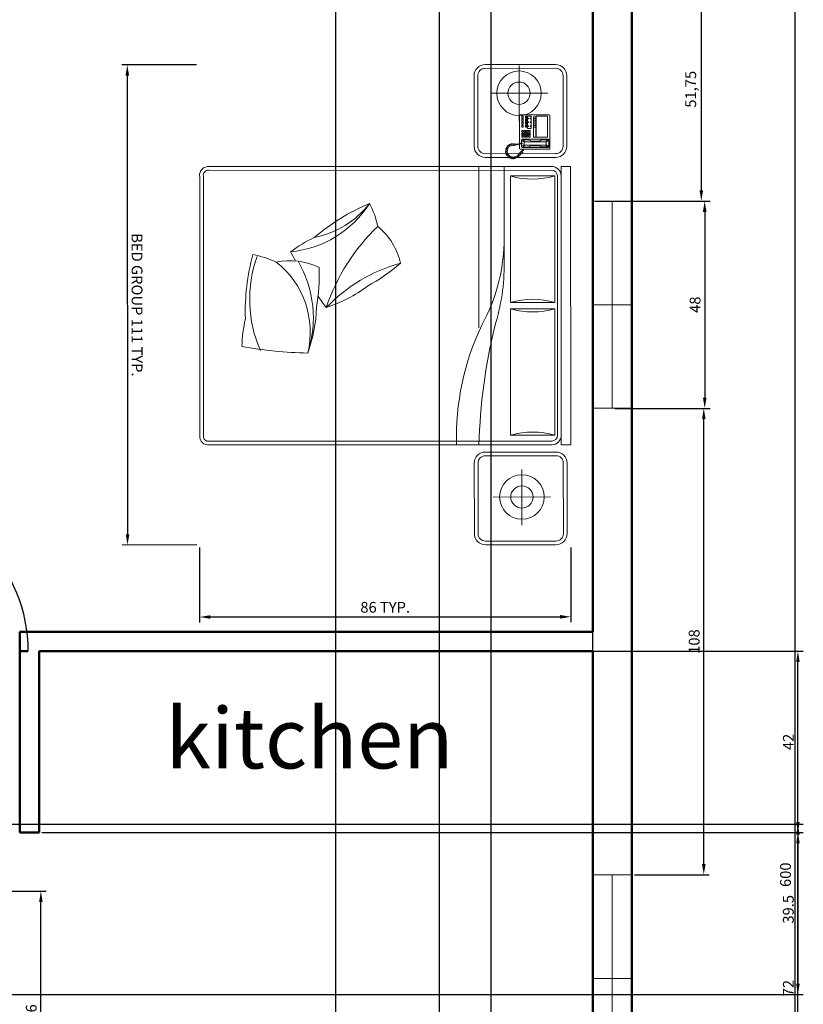
# Model space of a CAD drawing. Units: inches. Extents: x 907 to 2409, y 377 to 1163.
# Tile 7 of 9: x 1197 to 1378, y 687 to 915. Entities that reach past the tile are written whole.
import ezdxf

# ---------------------------------------------------------------- set-up
doc = ezdxf.new("R2010")
doc.units = ezdxf.units.IN
for name, color, linetype, lineweight in [('A-ANNO-DIMS', 2, 'Continuous', 18), ('A-AREA-IDEN', 7, 'Continuous', 18), ('A-DOOR', 3, 'Continuous', 25), ('A-FURN', 8, 'Continuous', 18), ('A-GLAZ', 4, 'Continuous', 18), ('A-WALL', 7, 'Continuous', 50)]:
    doc.layers.add(name, color=color, linetype=linetype, lineweight=lineweight)
doc.styles.get("Standard").update_dxf_attribs({"font": 'arial.ttf'})
doc.dimstyles.new('ISO-25', dxfattribs={"dimtxt": 2.5, "dimasz": 2.5, "dimexe": 1.25, "dimexo": 0.625, "dimtad": 1, "dimtxsty": 'Standard', "dimcen": 2.5, "dimadec": 0, "dimazin": 0, "dimtfac": 1, "dimtmove": 0, "dimatfit": 3, "dimfxl": 1, "dimarcsym": 0})

# ---------------------------------------------------------------- blocks, each defined once
blk = doc.blocks.new('A$C356F0359')
for p, q in [((0.4398, 1.9801), (0.0598, 1.9801)), ((0.5489, 2), (2.0492, 2)), ((0.5489, 1.9489), (0.5489, 2)), ((2.0492, 1.9489), (2.0492, 2)), ((2.5283, 1.9801), (2.1483, 1.9801)), ((-0.0002, 1.9201), (-0.0002, 1.5401)), ((0.0198, 1.9201), (0.0198, 1.5401)), ((0.4398, 1.9601), (0.0598, 1.9601)), ((0.4798, 1.5401), (0.4798, 1.9201)), ((0.4998, 1.5401), (0.4998, 1.9201)), ((2.0492, 1.9489), (0.5489, 1.9489)), ((1.998, 1.9289), (0.6001, 1.9289)), ((2.0883, 1.9201), (2.0883, 1.5401)), ((2.1083, 1.9201), (2.1083, 1.5401)), ((2.5283, 1.9601), (2.1483, 1.9601)), ((2.5683, 1.5401), (2.5683, 1.9201)), ((2.5883, 1.5401), (2.5883, 1.9201)), ((0.1539, 1.5681), (0.1539, 1.8777)), ((0.2725, 1.8879), (0.2702, 1.8856)), ((0.2702, 1.8856), (0.2702, 1.7279)), ((0.2725, 1.8879), (0.4531, 1.8879)), ((0.3913, 1.8753), (0.277, 1.8753)), ((0.277, 1.8753), (0.277, 1.8147)), ((0.3913, 1.8147), (0.3913, 1.8753)), ((0.4016, 1.8787), (0.4062, 1.8845)), ((0.4016, 1.7404), (0.4016, 1.8787)), ((0.4062, 1.881), (0.405, 1.8765)), ((0.405, 1.8765), (0.4153, 1.8662)), ((0.405, 1.8765), (0.405, 1.8456)), ((0.4062, 1.8845), (0.4405, 1.8845)), ((0.4108, 1.8833), (0.4062, 1.881)), ((0.4108, 1.8833), (0.4382, 1.8833)), ((0.4165, 1.8685), (0.4108, 1.8833)), ((0.4153, 1.8662), (0.4165, 1.8685)), ((0.4153, 1.8147), (0.4153, 1.8662)), ((0.4325, 1.8685), (0.4165, 1.8685)), ((0.4325, 1.8685), (0.4382, 1.8833)), ((0.4336, 1.8662), (0.4325, 1.8685)), ((0.4439, 1.8765), (0.4336, 1.8662)), ((0.4336, 1.8147), (0.4336, 1.8662)), ((0.4382, 1.8833), (0.4428, 1.881)), ((0.4405, 1.8845), (0.4462, 1.8787)), ((0.4428, 1.881), (0.4439, 1.8765)), ((0.4439, 1.8765), (0.4439, 1.8456)), ((0.4462, 1.8787), (0.4462, 1.7416)), ((0.4531, 1.8879), (0.4553, 1.8856)), ((0.4553, 1.8856), (0.4553, 1.7279)), ((0.5489, 1.8977), (0.5489, 0.0512)), ((0.5689, 1.8977), (0.5689, 0.0512)), ((2.0292, 0.0512), (2.0292, 1.8977)), ((2.0492, 0.0512), (2.0492, 1.8977)), ((2.3306, 1.5822), (2.3306, 1.8917)), ((0.277, 1.8147), (0.3913, 1.8147)), ((0.3913, 1.8125), (0.2816, 1.8125)), ((0.2816, 1.8125), (0.2816, 1.801)), ((0.2907, 1.8125), (0.2907, 1.801)), ((0.2999, 1.8125), (0.2999, 1.801)), ((0.309, 1.8125), (0.309, 1.801)), ((0.3182, 1.8125), (0.3182, 1.801)), ((0.3273, 1.8125), (0.3273, 1.801)), ((0.3365, 1.8125), (0.3365, 1.801)), ((0.3913, 1.801), (0.3913, 1.8125)), ((0.405, 1.8456), (0.4073, 1.8399)), ((0.4073, 1.8399), (0.4108, 1.8342)), ((0.4108, 1.8342), (0.4119, 1.8262)), ((0.4119, 1.8262), (0.4119, 1.8147)), ((0.4119, 1.793), (0.4119, 1.8147)), ((0.4153, 1.8147), (0.4153, 1.753)), ((0.4336, 1.8147), (0.4336, 1.753)), ((0.4382, 1.8342), (0.4371, 1.8262)), ((0.4371, 1.8262), (0.4371, 1.8147)), ((0.4371, 1.793), (0.4371, 1.8147)), ((0.4416, 1.8399), (0.4382, 1.8342)), ((0.4439, 1.8456), (0.4416, 1.8399)), ((0.277, 1.7885), (0.277, 1.7679)), ((0.3445, 1.7885), (0.277, 1.7885)), ((0.277, 1.7679), (0.3445, 1.7679)), ((0.2782, 1.7622), (0.2782, 1.7576)), ((0.2896, 1.7622), (0.2782, 1.7622)), ((0.2782, 1.7576), (0.2896, 1.7576)), ((0.2816, 1.801), (0.3913, 1.801)), ((0.2885, 1.7862), (0.2885, 1.7827)), ((0.2919, 1.7862), (0.2885, 1.7862)), ((0.2885, 1.7827), (0.2919, 1.7827)), ((0.2919, 1.7736), (0.2885, 1.7736)), ((0.2885, 1.7736), (0.2885, 1.7702)), ((0.2885, 1.7702), (0.2919, 1.7702)), ((0.2896, 1.7576), (0.2896, 1.7622)), ((0.2919, 1.7827), (0.2919, 1.7862)), ((0.2919, 1.7702), (0.2919, 1.7736)), ((0.2942, 1.7622), (0.2942, 1.7576)), ((0.3056, 1.7622), (0.2942, 1.7622)), ((0.2942, 1.7576), (0.3056, 1.7576)), ((0.3056, 1.7576), (0.3056, 1.7622)), ((0.3125, 1.7862), (0.309, 1.7862)), ((0.309, 1.7862), (0.309, 1.7827)), ((0.309, 1.7827), (0.3125, 1.7827)), ((0.3125, 1.7736), (0.309, 1.7736)), ((0.309, 1.7736), (0.309, 1.7702)), ((0.309, 1.7702), (0.3125, 1.7702)), ((0.3102, 1.7622), (0.3102, 1.7576)), ((0.3216, 1.7622), (0.3102, 1.7622)), ((0.3102, 1.7576), (0.3216, 1.7576)), ((0.3125, 1.7827), (0.3125, 1.7862)), ((0.3125, 1.7702), (0.3125, 1.7736)), ((0.3216, 1.7576), (0.3216, 1.7622)), ((0.3376, 1.7622), (0.3262, 1.7622)), ((0.3262, 1.7622), (0.3262, 1.7576)), ((0.3262, 1.7576), (0.3376, 1.7576)), ((0.333, 1.7862), (0.3296, 1.7862)), ((0.3296, 1.7862), (0.3296, 1.7827)), ((0.3296, 1.7827), (0.333, 1.7827)), ((0.333, 1.7736), (0.3296, 1.7736)), ((0.3296, 1.7736), (0.3296, 1.7702)), ((0.3296, 1.7702), (0.333, 1.7702)), ((0.333, 1.7827), (0.333, 1.7862)), ((0.333, 1.7702), (0.333, 1.7736)), ((0.3376, 1.7576), (0.3376, 1.7622)), ((0.3445, 1.7679), (0.3445, 1.7885)), ((0.3548, 1.7759), (0.3548, 1.7827)), ((0.3548, 1.7827), (0.3639, 1.7827)), ((0.3639, 1.7759), (0.3548, 1.7759)), ((0.3548, 1.7633), (0.3548, 1.7702)), ((0.3548, 1.7702), (0.3639, 1.7702)), ((0.3639, 1.7633), (0.3548, 1.7633)), ((0.3548, 1.7564), (0.3639, 1.7564)), ((0.3548, 1.7496), (0.3548, 1.7564)), ((0.3639, 1.7827), (0.3639, 1.7759)), ((0.3639, 1.7702), (0.3639, 1.7633)), ((0.3639, 1.7564), (0.3639, 1.7496)), ((0.3685, 1.7827), (0.3776, 1.7827)), ((0.3685, 1.7759), (0.3685, 1.7827)), ((0.3776, 1.7759), (0.3685, 1.7759)), ((0.3685, 1.7633), (0.3685, 1.7702)), ((0.3685, 1.7702), (0.3776, 1.7702)), ((0.3776, 1.7633), (0.3685, 1.7633)), ((0.3685, 1.7564), (0.3776, 1.7564)), ((0.3685, 1.7496), (0.3685, 1.7564)), ((0.3776, 1.7827), (0.3776, 1.7759)), ((0.3776, 1.7702), (0.3776, 1.7633)), ((0.3776, 1.7564), (0.3776, 1.7496)), ((0.3822, 1.7759), (0.3822, 1.7827)), ((0.3822, 1.7827), (0.3913, 1.7827)), ((0.3913, 1.7759), (0.3822, 1.7759)), ((0.3822, 1.7633), (0.3822, 1.7702)), ((0.3822, 1.7702), (0.3913, 1.7702)), ((0.3913, 1.7633), (0.3822, 1.7633)), ((0.3822, 1.7576), (0.3913, 1.7576)), ((0.3822, 1.7507), (0.3822, 1.7576)), ((0.3913, 1.7827), (0.3913, 1.7759)), ((0.3913, 1.7702), (0.3913, 1.7633)), ((0.3913, 1.7576), (0.3913, 1.7507)), ((0.405, 1.7736), (0.4073, 1.7793)), ((0.405, 1.7427), (0.405, 1.7736)), ((0.405, 1.7427), (0.4153, 1.753)), ((0.4073, 1.7793), (0.4108, 1.785)), ((0.4108, 1.785), (0.4119, 1.793)), ((0.4153, 1.753), (0.4165, 1.7507)), ((0.4336, 1.753), (0.4325, 1.7507)), ((0.4439, 1.7427), (0.4336, 1.753)), ((0.4382, 1.785), (0.4371, 1.793)), ((0.4416, 1.7793), (0.4382, 1.785)), ((0.4439, 1.7736), (0.4416, 1.7793)), ((0.4439, 1.7427), (0.4439, 1.7736)), ((0.3052, 1.7226), (0.0051, 1.7226)), ((0.2702, 1.7279), (0.2725, 1.7256)), ((0.4244, 1.7256), (0.2725, 1.7256)), ((0.2782, 1.745), (0.2896, 1.745)), ((0.2782, 1.7382), (0.2782, 1.745)), ((0.2896, 1.7382), (0.2782, 1.7382)), ((0.2896, 1.745), (0.2896, 1.7382)), ((0.2942, 1.745), (0.3056, 1.745)), ((0.2942, 1.7382), (0.2942, 1.745)), ((0.3056, 1.7382), (0.2942, 1.7382)), ((0.3056, 1.745), (0.3056, 1.7382)), ((0.3102, 1.745), (0.3216, 1.745)), ((0.3102, 1.7382), (0.3102, 1.745)), ((0.3216, 1.7382), (0.3102, 1.7382)), ((0.3216, 1.745), (0.3216, 1.7382)), ((0.3262, 1.7382), (0.3262, 1.745)), ((0.3262, 1.745), (0.3376, 1.745)), ((0.3376, 1.7382), (0.3262, 1.7382)), ((0.3376, 1.745), (0.3376, 1.7382)), ((0.3639, 1.7496), (0.3548, 1.7496)), ((0.3548, 1.737), (0.3548, 1.7439)), ((0.3548, 1.7439), (0.3639, 1.7439)), ((0.3639, 1.737), (0.3548, 1.737)), ((0.3639, 1.7439), (0.3639, 1.737)), ((0.3776, 1.7496), (0.3685, 1.7496)), ((0.3685, 1.737), (0.3685, 1.7439)), ((0.3685, 1.7439), (0.3776, 1.7439)), ((0.3776, 1.737), (0.3685, 1.737)), ((0.3776, 1.7439), (0.3776, 1.737)), ((0.3913, 1.7507), (0.3822, 1.7507)), ((0.3822, 1.7439), (0.3913, 1.7439)), ((0.3822, 1.737), (0.3822, 1.7439)), ((0.3913, 1.737), (0.3822, 1.737)), ((0.3913, 1.7439), (0.3913, 1.737)), ((0.4073, 1.7347), (0.4016, 1.7404)), ((0.4062, 1.7382), (0.405, 1.7427)), ((0.4108, 1.7359), (0.4062, 1.7382)), ((0.4234, 1.7347), (0.4073, 1.7347)), ((0.4165, 1.7507), (0.4108, 1.7359)), ((0.4108, 1.7359), (0.4234, 1.7359)), ((0.4325, 1.7507), (0.4165, 1.7507)), ((0.4233, 1.7393), (0.4235, 1.7294)), ((0.4268, 1.7393), (0.4233, 1.7393)), ((0.4235, 1.7294), (0.4263, 1.7179)), ((0.4263, 1.7179), (0.429, 1.707)), ((0.4274, 1.7301), (0.4268, 1.7393)), ((0.427, 1.7359), (0.4382, 1.7359)), ((0.4295, 1.6996), (0.427, 1.697)), ((0.4405, 1.7347), (0.4271, 1.7347)), ((0.429, 1.7227), (0.4274, 1.7301)), ((0.4531, 1.7256), (0.4284, 1.7256)), ((0.429, 1.707), (0.4288, 1.701)), ((0.4288, 1.701), (0.4295, 1.6996)), ((0.4318, 1.7119), (0.429, 1.7227)), ((0.4325, 1.7063), (0.4318, 1.7119)), ((0.4323, 1.7003), (0.4325, 1.7063)), ((0.4364, 1.6973), (0.4323, 1.7003)), ((0.4325, 1.7507), (0.4382, 1.7359)), ((0.4382, 1.7359), (0.4428, 1.7382)), ((0.4462, 1.7416), (0.4405, 1.7347)), ((0.4428, 1.7382), (0.4439, 1.7427)), ((0.4553, 1.7279), (0.4531, 1.7256)), ((0.4622, 1.7459), (0.4553, 1.7484)), ((0.4553, 1.7439), (0.4604, 1.7425)), ((0.4604, 1.7425), (0.465, 1.7388)), ((0.4654, 1.7427), (0.4622, 1.7459)), ((0.465, 1.7388), (0.4662, 1.7372)), ((0.4678, 1.7405), (0.4654, 1.7427)), ((0.4662, 1.7372), (0.4686, 1.7374)), ((0.4686, 1.7374), (0.4662, 1.735)), ((0.4662, 1.735), (0.4755, 1.7268)), ((0.4721, 1.7421), (0.4678, 1.7405)), ((0.4741, 1.7401), (0.4721, 1.7421)), ((0.4725, 1.7366), (0.4741, 1.7401)), ((0.4753, 1.7388), (0.4725, 1.7366)), ((0.4783, 1.7356), (0.4753, 1.7388)), ((0.4755, 1.7268), (0.4906, 1.7139)), ((0.4759, 1.729), (0.4783, 1.7356)), ((0.4821, 1.7322), (0.4759, 1.729)), ((0.4874, 1.7272), (0.4821, 1.7322)), ((0.4862, 1.7199), (0.4874, 1.7272)), ((0.4914, 1.7231), (0.4862, 1.7199)), ((0.4908, 1.7135), (0.4984, 1.6917)), ((0.4958, 1.7185), (0.4914, 1.7231)), ((0.494, 1.7135), (0.4958, 1.7185)), ((0.501, 1.7142), (0.494, 1.7135)), ((0.4964, 1.7047), (0.5031, 1.7072)), ((0.5038, 1.7049), (0.4964, 1.7047)), ((0.5005, 1.695), (0.5054, 1.6996)), ((0.5031, 1.7072), (0.501, 1.7142)), ((0.5054, 1.6996), (0.5038, 1.7049)), ((2.4819, 1.7366), (2.1818, 1.7366)), ((0.427, 1.697), (0.4265, 1.6915)), ((0.4265, 1.6915), (0.4332, 1.6903)), ((0.4332, 1.6903), (0.4267, 1.6864)), ((0.4267, 1.6864), (0.4272, 1.6801)), ((0.4272, 1.6801), (0.4346, 1.6794)), ((0.4346, 1.6794), (0.4281, 1.6744)), ((0.4281, 1.6744), (0.4311, 1.669)), ((0.4311, 1.669), (0.4381, 1.6704)), ((0.4381, 1.6704), (0.4348, 1.6639)), ((0.4348, 1.6639), (0.4383, 1.6598)), ((0.4355, 1.6919), (0.4364, 1.6973)), ((0.4367, 1.6774), (0.4355, 1.6919)), ((0.4455, 1.6663), (0.4367, 1.6774)), ((0.4383, 1.6598), (0.4436, 1.6637)), ((0.4436, 1.6637), (0.4427, 1.6575)), ((0.4427, 1.6575), (0.4471, 1.6547)), ((0.4577, 1.6598), (0.4455, 1.6663)), ((0.4471, 1.6547), (0.4526, 1.6593)), ((0.4526, 1.6593), (0.4519, 1.6517)), ((0.4519, 1.6517), (0.4568, 1.6503)), ((0.4568, 1.6503), (0.4598, 1.6565)), ((0.4716, 1.6586), (0.4577, 1.6598)), ((0.4598, 1.6565), (0.4626, 1.6503)), ((0.4626, 1.6503), (0.4665, 1.6498)), ((0.4665, 1.6498), (0.4681, 1.6565)), ((0.4681, 1.6565), (0.4707, 1.6491)), ((0.4707, 1.6491), (0.4751, 1.6503)), ((0.485, 1.6644), (0.4716, 1.6586)), ((0.4751, 1.6503), (0.4753, 1.6565)), ((0.4753, 1.6565), (0.4806, 1.6519)), ((0.4806, 1.6519), (0.4843, 1.6538)), ((0.4843, 1.6538), (0.4836, 1.6607)), ((0.4836, 1.6607), (0.4885, 1.6547)), ((0.4952, 1.6744), (0.485, 1.6644)), ((0.4885, 1.6547), (0.4922, 1.6579)), ((0.4922, 1.6579), (0.4894, 1.6642)), ((0.4894, 1.6642), (0.4959, 1.6614)), ((0.4984, 1.6917), (0.4952, 1.6744)), ((0.4957, 1.6704), (0.5024, 1.6683)), ((0.4989, 1.6642), (0.4957, 1.6704)), ((0.4959, 1.6614), (0.4989, 1.6642)), ((0.5042, 1.673), (0.4987, 1.6792)), ((0.4987, 1.6792), (0.5058, 1.679)), ((0.5068, 1.695), (0.5005, 1.695)), ((0.5008, 1.6871), (0.5079, 1.6892)), ((0.5068, 1.6836), (0.5008, 1.6871)), ((0.5024, 1.6683), (0.5042, 1.673)), ((0.5058, 1.679), (0.5068, 1.6836)), ((0.5079, 1.6892), (0.5068, 1.695)), ((0.0598, 1.5001), (0.4398, 1.5001)), ((2.1483, 1.5001), (2.5283, 1.5001)), ((0.0598, 1.4801), (0.4398, 1.4801)), ((2.1483, 1.4801), (2.5283, 1.4801)), ((0.6001, 0.02), (1.998, 0.02)), ((0.6001, 0), (1.998, 0))]:
    blk.add_line(p, q)
at = {"linetype": 'ByBlock'}
for p, q in [((0.6001, 1.9147), (1.282, 1.9147)), ((0.6001, 1.6759), (0.6001, 1.9147)), ((1.282, 1.9147), (1.282, 1.6759)), ((1.3161, 1.9147), (1.998, 1.9147)), ((1.3161, 1.6759), (1.3161, 1.9147)), ((1.998, 1.9147), (1.998, 1.6759)), ((1.282, 1.6759), (0.6001, 1.6759)), ((1.998, 1.6759), (1.3161, 1.6759)), ((1.0687, 1.6418), (0.5489, 1.6418)), ((1.4185, 1.5053), (0.5489, 1.5053))]:
    blk.add_line(p, q, dxfattribs=at)
for centre in [(0.1539, 1.7226), (2.3306, 1.7366)]:
    blk.add_circle(centre, 0.12, dxfattribs=at)
for centre in [(0.1539, 1.7226), (2.3306, 1.7366)]:
    blk.add_circle(centre, 0.06)
for centre, radius, start, end in [((0.0598, 1.9201), 0.06, 90, 180), ((0.4398, 1.9201), 0.06, 0, 90), ((2.1483, 1.9201), 0.06, 90, 180), ((2.5283, 1.9201), 0.06, 0, 90), ((0.0598, 1.9201), 0.04, 90, 180), ((0.4398, 1.9201), 0.04, 0, 90), ((0.6001, 1.8977), 0.0512, 90, 180), ((0.6001, 1.8977), 0.0312, 90, 180), ((1.998, 1.8977), 0.0512, 0, 90), ((1.998, 1.8977), 0.0312, 0, 90), ((2.1483, 1.9201), 0.04, 90, 180), ((2.5283, 1.9201), 0.04, 0, 90), ((0.0598, 1.5401), 0.06, 180, 270), ((0.0598, 1.5401), 0.04, 180, 270), ((0.4398, 1.5401), 0.04, 270, 0), ((0.4398, 1.5401), 0.06, 270, 0), ((2.1483, 1.5401), 0.06, 180, 270), ((2.1483, 1.5401), 0.04, 180, 270), ((2.5283, 1.5401), 0.06, 270, 0), ((2.5283, 1.5401), 0.04, 270, 0), ((1.1471, 0.7332), 0.3575, 102.4782, 140.4625), ((1.9086, 1.3124), 0.8697, 195.336, 226.4193), ((0.3249, 0.4335), 0.9879, 28.4971, 41.0566), ((0.9965, 0.4273), 0.548, 103.2034, 117.0362), ((1.6529, 1.7059), 1.0798, 223.6306, 251.4288), ((0.4451, 0.4375), 0.5655, 5.3391, 57.6895), ((0.4517, 0.5274), 0.4879, 10.6986, 52.6864), ((1.8195, 1.3719), 1.1652, 203.0642, 220.3209), ((0.5617, 0.4344), 0.7874, 18.3527, 36.6851), ((1.4135, 0.487), 0.3575, 154.0418, 192.0262), ((1.1372, -0.3434), 0.9879, 80.0607, 92.6202), ((-0.021, 2.4319), 2.1977, 305.2966, 307.2418), ((1.5949, 0.9312), 0.734, 205.259, 216.9351), ((1.3641, 0.0041), 0.6085, 71.81, 120.1351), ((1.44, 0.1186), 0.4774, 76.1849, 142.0017), ((1.2836, -0.1573), 0.7874, 69.9163, 88.2487), ((-0.6432, 0.628), 2.1977, 349.4884, 358.8054), ((-0.021, 2.4319), 2.1977, 297.9248, 299.3793), ((1.5595, 0.1789), 0.548, 154.767, 168.5998), ((1.2647, 0.9578), 0.6885, 250.2936, 293.6414), ((1.3312, 1.4107), 1.1652, 254.6278, 271.8845), ((1.5368, 0.9609), 0.734, 256.8226, 268.4988), ((0.5943, 0.0454), 0.0458, 172.7599, 277.2401), ((0.5943, 0.0454), 0.0258, 172.7599, 277.2401), ((2.0038, 0.0454), 0.0458, 262.7599, 7.2401), ((2.0038, 0.0454), 0.0258, 262.7599, 7.2401)]:
    blk.add_arc(centre, radius, start, end)
for centre, radius, start, end in [((0.1906, 1.7953), 0.4265, 343.7398, 16.2602), ((1.6914, 1.7953), 0.4265, 163.7398, 196.2602), ((0.9067, 1.7953), 0.4265, 343.7398, 16.2602), ((2.4075, 1.7953), 0.4265, 163.7398, 196.2602), ((0.9303, 0.657), 0.9853, 61.4328, 88.1261), ((1.0826, 0.5712), 1.0706, 72.1966, 90.7418), ((2.1368, 4.5996), 3.0955, 256.4201, 268.3789), ((2.0056, 2.7745), 1.3903, 244.2427, 271.7984)]:
    blk.add_arc(centre, radius, start, end, dxfattribs=at)
blk = doc.blocks.new('*D16')
at = {"layer": 'A-ANNO-DIMS', "color": 0, "lineweight": -2, "transparency": 16777216}
for p, q in [((1330.24, 924.62), (1355.99, 924.62)), ((1354.74, 922.12), (1354.74, 875.37)), ((1330.24, 872.87), (1355.99, 872.87))]:
    blk.add_line(p, q, dxfattribs=at)
at = {"layer": 'A-ANNO-DIMS', "color": 0, "transparency": 16777216}
for points in [[(1354.32, 922.12), (1355.16, 922.12), (1354.74, 924.62)], [(1354.32, 875.37), (1355.16, 875.37), (1354.74, 872.87)]]:
    blk.add_solid(points, dxfattribs=at)
at = {"layer": 'Defpoints', "color": 0, "transparency": 16777216}
for p in [(1329.61, 924.62), (1329.61, 872.87), (1354.74, 872.87)]:
    blk.add_point(p, dxfattribs=at)
at = {"layer": 'A-ANNO-DIMS', "color": 0, "transparency": 16777216, "insert": (1352.61, 898.75), "char_height": 2.5, "attachment_point": 5, "rotation": 90}
blk.add_mtext('51,75', dxfattribs=at)
blk = doc.blocks.new('*D17')
at = {"layer": 'A-ANNO-DIMS', "color": 0, "lineweight": -2, "transparency": 16777216}
for p, q in [((1334.74, 872.87), (1356.77, 872.87)), ((1355.52, 870.37), (1355.52, 827.37)), ((1334.74, 824.87), (1356.77, 824.87))]:
    blk.add_line(p, q, dxfattribs=at)
at = {"layer": 'A-ANNO-DIMS', "color": 0, "transparency": 16777216}
for points in [[(1355.11, 870.37), (1355.94, 870.37), (1355.52, 872.87)], [(1355.11, 827.37), (1355.94, 827.37), (1355.52, 824.87)]]:
    blk.add_solid(points, dxfattribs=at)
at = {"layer": 'Defpoints', "color": 0, "transparency": 16777216}
for p in [(1334.11, 872.87), (1334.11, 824.87), (1355.52, 824.87)]:
    blk.add_point(p, dxfattribs=at)
at = {"layer": 'A-ANNO-DIMS', "color": 0, "transparency": 16777216, "insert": (1353.62, 848.87), "char_height": 2.5, "attachment_point": 5, "rotation": 90}
blk.add_mtext('48', dxfattribs=at)
blk = doc.blocks.new('*D18')
at = {"layer": 'A-ANNO-DIMS', "color": 0, "lineweight": -2, "transparency": 16777216}
for p, q in [((1339.24, 824.87), (1356.56, 824.87)), ((1355.31, 719.37), (1355.31, 822.37)), ((1339.24, 716.87), (1356.56, 716.87))]:
    blk.add_line(p, q, dxfattribs=at)
at = {"layer": 'A-ANNO-DIMS', "color": 0, "transparency": 16777216}
for points in [[(1354.9, 822.37), (1355.73, 822.37), (1355.31, 824.87)], [(1354.9, 719.37), (1355.73, 719.37), (1355.31, 716.87)]]:
    blk.add_solid(points, dxfattribs=at)
at = {"layer": 'Defpoints', "color": 0, "transparency": 16777216}
for p in [(1338.61, 824.87), (1355.31, 824.87), (1338.61, 716.87)]:
    blk.add_point(p, dxfattribs=at)
at = {"layer": 'A-ANNO-DIMS', "color": 0, "transparency": 16777216, "insert": (1353.41, 770.87), "char_height": 2.5, "attachment_point": 5, "rotation": 90}
blk.add_mtext('108', dxfattribs=at)
blk = doc.blocks.new('*D20')
at = {"layer": 'A-ANNO-DIMS', "color": 0, "lineweight": -2, "transparency": 16777216}
for p, q in [((1339.24, 1016.87), (1377.72, 1016.87)), ((1376.47, 419.37), (1376.47, 1014.37)), ((1339.24, 416.87), (1377.72, 416.87))]:
    blk.add_line(p, q, dxfattribs=at)
at = {"layer": 'A-ANNO-DIMS', "color": 0, "transparency": 16777216}
for points in [[(1376.05, 1014.37), (1376.88, 1014.37), (1376.47, 1016.87)], [(1376.05, 419.37), (1376.88, 419.37), (1376.47, 416.87)]]:
    blk.add_solid(points, dxfattribs=at)
at = {"layer": 'Defpoints', "color": 0, "transparency": 16777216}
for p in [(1338.61, 1016.87), (1376.47, 1016.87), (1338.61, 416.87)]:
    blk.add_point(p, dxfattribs=at)
at = {"layer": 'A-ANNO-DIMS', "color": 0, "transparency": 16777216, "insert": (1374.56, 716.87), "char_height": 2.5, "attachment_point": 5, "rotation": 90}
blk.add_mtext('600', dxfattribs=at)
blk = doc.blocks.new('DOOR-36IN')
for p, q in [((36, 36), (36, 0)), ((36, 0), (34, 0)), ((36, 0), (34, 0))]:
    blk.add_line(p, q)
blk.add_lwpolyline([(36, 36), (34, 36), (34, 0), (36, 0)], close=True)
blk.add_arc((36.06, 0), 36.06, 93.2732, 180)
blk = doc.blocks.new('WIN-48IN')
for p, q in [((9, 48), (0, 48)), ((4.5, 48), (4.5, 0)), ((9, 24), (0, 24)), ((9, 0), (0, 0))]:
    blk.add_line(p, q)
blk = doc.blocks.new('*D51')
at = {"layer": 'A-ANNO-DIMS', "color": 0, "lineweight": -2, "transparency": 16777216}
for p, q in [((1237.83, 904.42), (1220.53, 904.41)), ((1221.78, 901.91), (1221.84, 795.72)), ((1237.9, 793.23), (1220.59, 793.22))]:
    blk.add_line(p, q, dxfattribs=at)
at = {"layer": 'A-ANNO-DIMS', "color": 0, "transparency": 16777216}
for points in [[(1222.2, 901.91), (1221.37, 901.91), (1221.78, 904.41)], [(1222.26, 795.72), (1221.43, 795.72), (1221.84, 793.22)]]:
    blk.add_solid(points, dxfattribs=at)
at = {"layer": 'Defpoints', "color": 0, "transparency": 16777216}
for p in [(1238.46, 904.42), (1221.84, 793.22), (1238.52, 793.23)]:
    blk.add_point(p, dxfattribs=at)
at = {"layer": 'A-ANNO-DIMS', "color": 0, "transparency": 16777216, "insert": (1223.73, 848.82), "char_height": 2.5, "attachment_point": 5, "rotation": 270.0319}
blk.add_mtext('BED GROUP 111 TYP.', dxfattribs=at)
blk = doc.blocks.new('*D52')
at = {"layer": 'A-ANNO-DIMS', "color": 0, "lineweight": -2, "transparency": 16777216}
for p, q in [((1238.52, 792.61), (1238.53, 775.3)), ((1324.5, 792.65), (1324.51, 775.35)), ((1241.03, 776.56), (1322.01, 776.6))]:
    blk.add_line(p, q, dxfattribs=at)
at = {"layer": 'A-ANNO-DIMS', "color": 0, "transparency": 16777216}
for points in [[(1241.03, 776.97), (1241.03, 776.14), (1238.53, 776.55)], [(1322.01, 777.02), (1322.01, 776.18), (1324.51, 776.6)]]:
    blk.add_solid(points, dxfattribs=at)
at = {"layer": 'Defpoints', "color": 0, "transparency": 16777216}
for p in [(1238.52, 793.23), (1324.5, 793.28), (1324.51, 776.6)]:
    blk.add_point(p, dxfattribs=at)
at = {"layer": 'A-ANNO-DIMS', "color": 0, "transparency": 16777216, "insert": (1281.52, 778.48), "char_height": 2.5, "attachment_point": 5, "rotation": 0.0319}
blk.add_mtext('86 TYP.', dxfattribs=at)
blk = doc.blocks.new('*D58')
at = {"layer": 'A-ANNO-DIMS', "color": 0, "lineweight": -2, "transparency": 16777216}
for p, q in [((1191.96, 713.06), (1203.02, 713.06)), ((1201.77, 659.4), (1201.77, 710.56)), ((1191.96, 656.9), (1203.02, 656.9))]:
    blk.add_line(p, q, dxfattribs=at)
at = {"layer": 'A-ANNO-DIMS', "color": 0, "transparency": 16777216}
for points in [[(1201.36, 710.56), (1202.19, 710.56), (1201.77, 713.06)], [(1201.36, 659.4), (1202.19, 659.4), (1201.77, 656.9)]]:
    blk.add_solid(points, dxfattribs=at)
at = {"layer": 'Defpoints', "color": 0, "transparency": 16777216}
for p in [(1191.34, 713.06), (1201.77, 713.06), (1191.34, 656.9)]:
    blk.add_point(p, dxfattribs=at)
at = {"layer": 'A-ANNO-DIMS', "color": 0, "transparency": 16777216, "insert": (1199.87, 684.98), "char_height": 2.5, "attachment_point": 5, "rotation": 90}
blk.add_mtext('56', dxfattribs=at)
blk = doc.blocks.new('*D73')
at = {"layer": 'A-ANNO-DIMS', "color": 0, "lineweight": -2, "transparency": 16777216}
for p, q in [((1201.97, 768.62), (1378.36, 768.62)), ((1377.11, 729.12), (1377.11, 766.12)), ((1201.97, 726.62), (1378.36, 726.62))]:
    blk.add_line(p, q, dxfattribs=at)
at = {"layer": 'A-ANNO-DIMS', "color": 0, "transparency": 16777216}
for points in [[(1376.7, 766.12), (1377.53, 766.12), (1377.11, 768.62)], [(1376.7, 729.12), (1377.53, 729.12), (1377.11, 726.62)]]:
    blk.add_solid(points, dxfattribs=at)
at = {"layer": 'Defpoints', "color": 0, "transparency": 16777216}
for p in [(1201.34, 768.62), (1377.11, 768.62), (1201.34, 726.62)]:
    blk.add_point(p, dxfattribs=at)
at = {"layer": 'A-ANNO-DIMS', "color": 0, "transparency": 16777216, "insert": (1375.23, 747.62), "char_height": 2.5, "attachment_point": 5, "rotation": 90}
blk.add_mtext('42', dxfattribs=at)
blk = doc.blocks.new('*D74')
at = {"layer": 'A-ANNO-DIMS', "color": 0, "lineweight": -2, "transparency": 16777216}
for p, q in [((1201.97, 726.62), (1378.36, 726.62)), ((1377.11, 657.12), (1377.11, 724.12)), ((1201.97, 654.62), (1378.36, 654.62))]:
    blk.add_line(p, q, dxfattribs=at)
at = {"layer": 'A-ANNO-DIMS', "color": 0, "transparency": 16777216}
for points in [[(1376.7, 724.12), (1377.53, 724.12), (1377.11, 726.62)], [(1376.7, 657.12), (1377.53, 657.12), (1377.11, 654.62)]]:
    blk.add_solid(points, dxfattribs=at)
at = {"layer": 'Defpoints', "color": 0, "transparency": 16777216}
for p in [(1201.34, 726.62), (1377.11, 726.62), (1201.34, 654.62)]:
    blk.add_point(p, dxfattribs=at)
at = {"layer": 'A-ANNO-DIMS', "color": 0, "transparency": 16777216, "insert": (1375.23, 690.62), "char_height": 2.5, "attachment_point": 5, "rotation": 90}
blk.add_mtext('72', dxfattribs=at)
blk = doc.blocks.new('*D77')
at = {"layer": 'A-ANNO-DIMS', "color": 0, "lineweight": -2, "transparency": 16777216}
for p, q in [((1270.1, 534.51), (1270.1, 1056.62)), ((1294.1, 534.51), (1294.1, 1056.62)), ((1272.6, 1055.37), (1291.6, 1055.37))]:
    blk.add_line(p, q, dxfattribs=at)
at = {"layer": 'A-ANNO-DIMS', "color": 0, "transparency": 16777216}
for points in [[(1272.6, 1055.79), (1272.6, 1054.95), (1270.1, 1055.37)], [(1291.6, 1055.79), (1291.6, 1054.95), (1294.1, 1055.37)]]:
    blk.add_solid(points, dxfattribs=at)
at = {"layer": 'Defpoints', "color": 0, "transparency": 16777216}
for p in [(1294.1, 1055.37), (1270.1, 533.88), (1294.1, 533.88)]:
    blk.add_point(p, dxfattribs=at)
at = {"layer": 'A-ANNO-DIMS', "color": 0, "transparency": 16777216, "insert": (1282.1, 1057.25), "char_height": 2.5, "attachment_point": 5}
blk.add_mtext('24', dxfattribs=at)
blk = doc.blocks.new('*D78')
at = {"layer": 'A-ANNO-DIMS', "color": 0, "lineweight": -2, "transparency": 16777216}
for p, q in [((1306.1, 534.51), (1306.1, 1056.62)), ((1329.61, 534.51), (1329.61, 1056.62)), ((1308.6, 1055.37), (1327.11, 1055.37))]:
    blk.add_line(p, q, dxfattribs=at)
at = {"layer": 'A-ANNO-DIMS', "color": 0, "transparency": 16777216}
for points in [[(1308.6, 1055.79), (1308.6, 1054.95), (1306.1, 1055.37)], [(1327.11, 1055.79), (1327.11, 1054.95), (1329.61, 1055.37)]]:
    blk.add_solid(points, dxfattribs=at)
at = {"layer": 'Defpoints', "color": 0, "transparency": 16777216}
for p in [(1329.61, 1055.37), (1306.1, 533.88), (1329.61, 533.88)]:
    blk.add_point(p, dxfattribs=at)
at = {"layer": 'A-ANNO-DIMS', "color": 0, "transparency": 16777216, "insert": (1317.86, 1057.27), "char_height": 2.5, "attachment_point": 5}
blk.add_mtext('23.514', dxfattribs=at)
blk = doc.blocks.new('*D81')
at = {"layer": 'A-ANNO-DIMS', "color": 0, "lineweight": -2, "transparency": 16777216}
for p, q in [((1053.49, 728.62), (1378.36, 728.62)), ((1377.11, 726.12), (1377.11, 691.62)), ((1048.99, 689.12), (1378.36, 689.12))]:
    blk.add_line(p, q, dxfattribs=at)
at = {"layer": 'A-ANNO-DIMS', "color": 0, "transparency": 16777216}
for points in [[(1376.7, 726.12), (1377.53, 726.12), (1377.11, 728.62)], [(1376.7, 691.62), (1377.53, 691.62), (1377.11, 689.12)]]:
    blk.add_solid(points, dxfattribs=at)
at = {"layer": 'Defpoints', "color": 0, "transparency": 16777216}
for p in [(1052.86, 728.62), (1048.36, 689.12), (1377.11, 689.12)]:
    blk.add_point(p, dxfattribs=at)
at = {"layer": 'A-ANNO-DIMS', "color": 0, "transparency": 16777216, "insert": (1375.21, 708.87), "char_height": 2.5, "attachment_point": 5, "rotation": 90}
blk.add_mtext('39.5', dxfattribs=at)

msp = doc.modelspace()

# ---------------------------------------------------------------- linework, layer by layer
at = {"layer": 'A-WALL'}
for p, q in [((1338.6122, 416.8705), (1338.6122, 1016.8705)), ((1338.6122, 416.8705), (1338.6122, 1016.8705)), ((1329.6122, 773.1205), (1329.6122, 924.6205)), ((1196.8622, 773.08), (1198.4767, 773.1205)), ((1196.8622, 768.6205), (1196.8622, 773.08)), ((1198.4767, 773.1205), (1329.6122, 773.1205)), ((1198.4818, 773.08), (1199.4225, 773.08)), ((1338.6122, 770.8705), (1338.6122, 614.8705)), ((1196.8622, 768.6205), (1196.8622, 726.6205)), ((1196.8622, 768.6205), (1198.7586, 768.6205)), ((1201.3421, 768.6205), (1201.3421, 726.6205)), ((1201.3421, 768.6205), (1329.6122, 768.6205)), ((1329.6122, 617.1205), (1329.6122, 768.6205)), ((1196.8622, 726.6205), (1201.3421, 726.6205))]:
    msp.add_line(p, q, dxfattribs=at)
msp.add_lwpolyline([(1216.3622, 416.8705), (1338.6122, 416.8705), (1338.6122, 1016.8705), (978.6122, 1016.8705), (978.6122, 416.8705), (1100.8622, 416.8705)], dxfattribs=at)

# ---------------------------------------------------------------- block references
at = {"layer": 'A-DOOR', "extrusion": (0, 0, -1), "zscale": -1}
msp.add_blockref('DOOR-36IN', (-1198.7586, 768.6205), dxfattribs=at)
at = {"layer": 'A-FURN', "xscale": 42.95257138859579, "yscale": 42.95257138859579, "zscale": 42.95257138859579, "rotation": 270.0319484166595}
msp.add_blockref('A$C356F0359', (1238.5348, 904.4063), dxfattribs=at)
at = {"layer": 'A-GLAZ'}
for p in [(1329.612, 824.871), (1329.612, 668.871)]:
    msp.add_blockref('WIN-48IN', p, dxfattribs=at)

# ---------------------------------------------------------------- texts
at = {"layer": 'A-AREA-IDEN', "insert": (1230.6297, 755.516), "char_height": 14.02836, "attachment_point": 1}
msp.add_mtext_dynamic_manual_height_columns('kitchen', width=7.730354, gutter_width=70.1418, heights=[0], dxfattribs=at)

# ---------------------------------------------------------------- dimensions: what is measured, and where the dimension line sits
at = {"layer": 'A-ANNO-DIMS'}
for base, p1, p2, override, picture, middle in [((1294.0979, 1055.3705), (1270.0979, 533.8833), (1294.0979, 533.8833), {"dimdec": 0, "dimlfac": 1, "dimrnd": 0, "dimzin": 0, "dimdsep": 46, "dimlunit": 2}, '*D77', (1282.0979, 1057.2507)), ((1329.6122, 1055.3705), (1306.0979, 533.8833), (1329.6122, 533.8833), {"dimdec": 3, "dimlfac": 1, "dimrnd": 0, "dimzin": 0, "dimdsep": 46, "dimlunit": 2}, '*D78', (1317.8551, 1057.2728))]:
    dim = msp.add_linear_dim(base=base, p1=p1, p2=p2, dimstyle='ISO-25', override=override, dxfattribs=at)
    dim.commit()
    dim.dimension.update_dxf_attribs({"geometry": picture, "text_midpoint": middle})
for base, p1, p2, override, picture, middle in [((1376.4651, 1016.8705), (1338.6122, 416.8705), (1338.6122, 1016.8705), {"dimclrd": 0, "dimclre": 0, "dimclrt": 0}, '*D20', (1374.5637, 716.8705)), ((1354.7405, 872.8705), (1329.6122, 924.6205), (1329.6122, 872.8705), {"dimclrd": 0, "dimclre": 0, "dimclrt": 0}, '*D16', (1352.6131, 898.7455)), ((1355.5232, 824.8705), (1334.1122, 872.8705), (1334.1122, 824.8705), {"dimclrd": 0, "dimclre": 0, "dimclrt": 0}, '*D17', (1353.6218, 848.8705)), ((1355.3149, 824.8705), (1338.6122, 716.8705), (1338.6122, 824.8705), {"dimclrd": 0, "dimclre": 0, "dimclrt": 0}, '*D18', (1353.4135, 770.8705)), ((1377.1122, 768.6205), (1201.3421, 726.6205), (1201.3421, 768.6205), {"dimdec": 0, "dimlfac": 1, "dimrnd": 0, "dimzin": 0, "dimdsep": 46, "dimlunit": 2}, '*D73', (1375.2321, 747.6205)), ((1377.1122, 689.1205), (1052.8622, 728.6205), (1048.3622, 689.1205), {"dimdec": 1, "dimlfac": 1, "dimrnd": 0, "dimzin": 0, "dimdsep": 46, "dimlunit": 2}, '*D81', (1375.2099, 708.8705)), ((1377.1122, 726.6205), (1201.3421, 654.6205), (1201.3421, 726.6205), {"dimdec": 0, "dimlfac": 1, "dimrnd": 0, "dimzin": 0, "dimdsep": 46, "dimlunit": 2}, '*D74', (1375.2321, 690.6205)), ((1201.775, 713.0624), (1191.3372, 656.8985), (1191.3372, 713.0624), {"dimdec": 0, "dimlfac": 1, "dimrnd": 0, "dimzin": 0, "dimdsep": 46, "dimlunit": 2}, '*D58', (1199.8735, 684.9804))]:
    dim = msp.add_linear_dim(base=base, p1=p1, p2=p2, angle=90, dimstyle='ISO-25', override=override, dxfattribs=at)
    dim.commit()
    dim.dimension.update_dxf_attribs({"geometry": picture, "text_midpoint": middle})
for base, p1, p2, angle, text, picture, middle in [((1221.8441, 793.2222), (1238.4598, 904.4159), (1238.5218, 793.2315), 270.031948, 'BED GROUP <> TYP.', '*D51', (1223.7316, 848.8155)), ((1324.5128, 776.6017), (1238.5218, 793.2315), (1324.5036, 793.2794), 0.031948, '<> TYP.', '*D52', (1281.5209, 778.4792))]:
    dim = msp.add_linear_dim(base=base, p1=p1, p2=p2, angle=angle, text=text, dimstyle='ISO-25', override={"dimdec": 0, "dimlfac": 1, "dimrnd": 0, "dimzin": 0, "dimdsep": 46, "dimlunit": 2}, dxfattribs=at)
    dim.commit()
    dim.dimension.update_dxf_attribs({"geometry": picture, "text_midpoint": middle})

doc.saveas('drawing.dxf')
